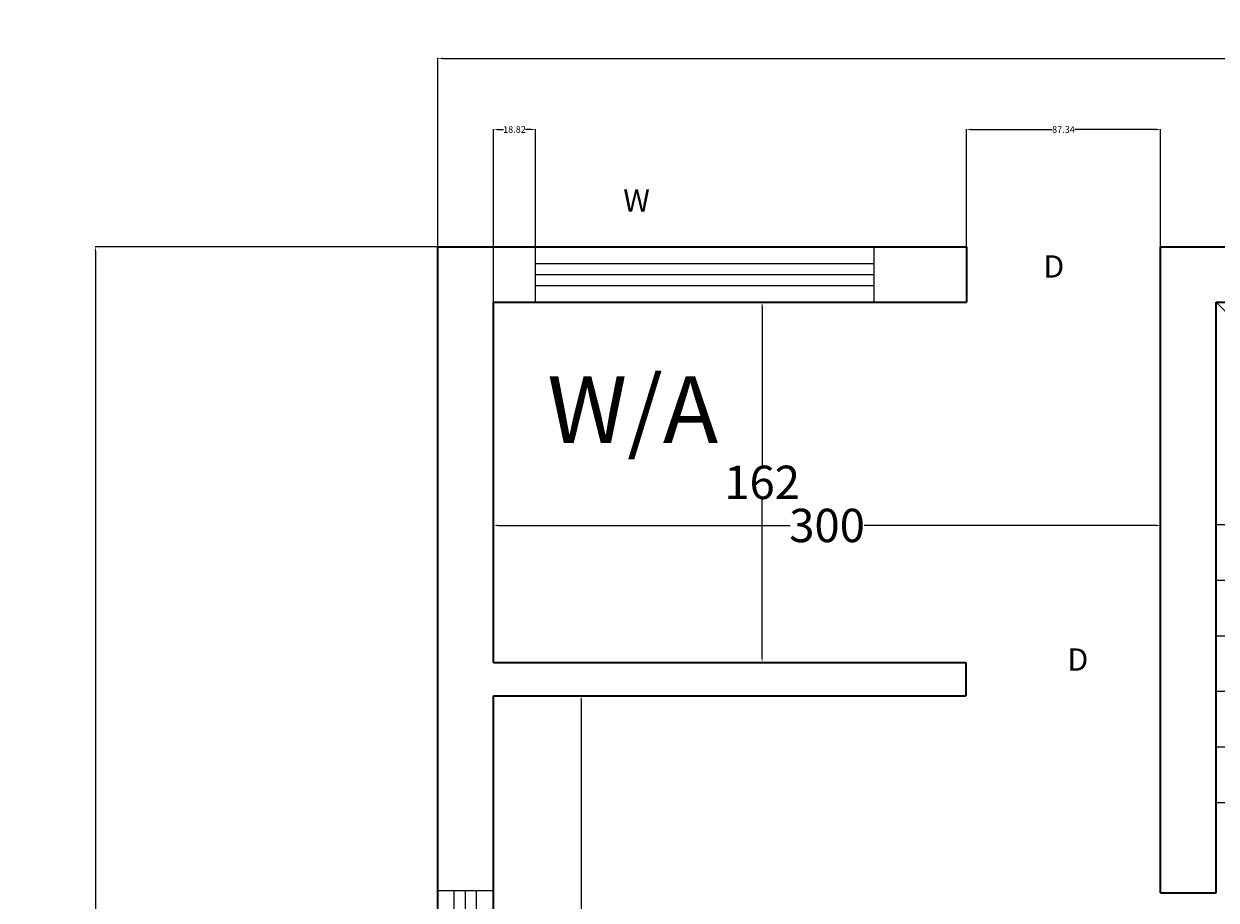
# Model space of a CAD drawing. Units: centimetres. Extents: x -121 to 3851, y -16 to 1180.
# Tile 4 of 16: x -121 to 415, y 586 to 980. Entities that reach past the tile are written whole.
import ezdxf

# ---------------------------------------------------------------- set-up
doc = ezdxf.new("R2010")
doc.units = ezdxf.units.CM
doc.header["$MEASUREMENT"] = 0
for name, color, linetype, lineweight in [('A-ANNO-DIMS', 2, 'Continuous', 18), ('A-ANNO-IDEN', 3, 'Continuous', 13), ('A-AREA-IDEN', 3, 'Continuous', 18), ('A-FLOR-STRS', 3, 'Continuous', 18), ('A-GLAZ', 4, 'Continuous', 18), ('A-WALL', 7, 'Continuous', 35)]:
    doc.layers.add(name, color=color, linetype=linetype, lineweight=lineweight)
doc.styles.get("Standard").update_dxf_attribs({"font": 'arial.ttf'})
doc.dimstyles.get("Standard").update_dxf_attribs({"dimtxt": 3, "dimasz": 2, "dimexe": 0.18, "dimexo": 0.0625, "dimgap": 0.09, "dimtad": 0, "dimtih": 1, "dimtoh": 1, "dimdec": 0, "dimzin": 0, "dimdsep": 46, "dimtxsty": 'Standard', "dimcen": 0.09, "dimadec": 0, "dimazin": 0, "dimtfac": 1, "dimtdec": 0, "dimtofl": 0, "dimtmove": 0, "dimatfit": 3, "dimfxl": 1, "dimtolj": 1, "dimtzin": 0, "dimarcsym": 0})

# ---------------------------------------------------------------- blocks, each defined once
blk = doc.blocks.new('*D1')
at = {"layer": 'A-ANNO-DIMS', "color": 0, "lineweight": -2, "transparency": 16777216}
for p, q in [((65.04, 880.08), (65.04, 964.95)), ((67.04, 964.77), (699.58, 964.77)), ((1419.04, 964.77), (786.5, 964.77)), ((1421.04, 880.08), (1421.04, 964.95))]:
    blk.add_line(p, q, dxfattribs=at)
at = {"layer": 'A-ANNO-DIMS', "color": 0, "transparency": 16777216}
for points in [[(67.04, 965.1), (67.04, 964.43), (65.04, 964.77)], [(1419.04, 965.1), (1419.04, 964.43), (1421.04, 964.77)]]:
    blk.add_solid(points, dxfattribs=at)
at = {"layer": 'Defpoints', "color": 0, "transparency": 16777216}
for p in [(1421.04, 964.77), (65.04, 880.01), (1421.04, 880.01)]:
    blk.add_point(p, dxfattribs=at)
at = {"layer": 'A-ANNO-DIMS', "color": 0, "transparency": 16777216, "insert": (743.04, 964.77), "char_height": 3, "attachment_point": 5}
blk.add_mtext('\\A1;{\\H10x;1356}', dxfattribs=at)
blk = doc.blocks.new('*D2')
at = {"layer": 'A-ANNO-DIMS', "color": 0, "lineweight": -2, "transparency": 16777216}
for p, q in [((64.98, 880.01), (-89.22, 880.01)), ((-89.04, 878.01), (-89.04, 487.42)), ((-89.04, 66.01), (-89.04, 456.61)), ((64.98, 64.01), (-89.22, 64.01))]:
    blk.add_line(p, q, dxfattribs=at)
at = {"layer": 'A-ANNO-DIMS', "color": 0, "transparency": 16777216}
for points in [[(-89.37, 878.01), (-88.71, 878.01), (-89.04, 880.01)], [(-89.37, 66.01), (-88.71, 66.01), (-89.04, 64.01)]]:
    blk.add_solid(points, dxfattribs=at)
at = {"layer": 'Defpoints', "color": 0, "transparency": 16777216}
for p in [(65.04, 880.01), (-89.04, 64.01), (65.04, 64.01)]:
    blk.add_point(p, dxfattribs=at)
at = {"layer": 'A-ANNO-DIMS', "color": 0, "transparency": 16777216, "insert": (-89.04, 472.01), "char_height": 3, "attachment_point": 5}
blk.add_mtext('\\A1;{\\H10x;816}', dxfattribs=at)
blk = doc.blocks.new('*D3')
at = {"layer": 'A-ANNO-DIMS', "color": 0, "lineweight": -2, "transparency": 16777216}
for p, q in [((185.01, 855.01), (211, 855.01)), ((210.82, 853.01), (210.82, 781.76)), ((210.82, 695.01), (210.82, 766.27)), ((185.01, 693.01), (211, 693.01))]:
    blk.add_line(p, q, dxfattribs=at)
at = {"layer": 'A-ANNO-DIMS', "color": 0, "transparency": 16777216}
for points in [[(210.48, 853.01), (211.15, 853.01), (210.82, 855.01)], [(210.48, 695.01), (211.15, 695.01), (210.82, 693.01)]]:
    blk.add_solid(points, dxfattribs=at)
at = {"layer": 'Defpoints', "color": 0, "transparency": 16777216}
for p in [(184.95, 855.01), (184.95, 693.01), (210.82, 693.01)]:
    blk.add_point(p, dxfattribs=at)
at = {"layer": 'A-ANNO-DIMS', "color": 0, "transparency": 16777216, "insert": (210.82, 774.01), "char_height": 3, "attachment_point": 5}
blk.add_mtext('\\A1;{\\H5x;162}', dxfattribs=at)
blk = doc.blocks.new('*D4')
at = {"layer": 'A-ANNO-DIMS', "color": 0, "lineweight": -2, "transparency": 16777216}
for p, q in [((90.04, 754.68), (90.04, 754.8)), ((92.04, 754.62), (223.41, 754.62)), ((388.04, 754.62), (256.67, 754.62)), ((390.04, 754.68), (390.04, 754.8))]:
    blk.add_line(p, q, dxfattribs=at)
at = {"layer": 'A-ANNO-DIMS', "color": 0, "transparency": 16777216}
for points in [[(92.04, 754.95), (92.04, 754.29), (90.04, 754.62)], [(388.04, 754.95), (388.04, 754.29), (390.04, 754.62)]]:
    blk.add_solid(points, dxfattribs=at)
at = {"layer": 'Defpoints', "color": 0, "transparency": 16777216}
for p in [(90.04, 754.62), (390.04, 754.62), (390.04, 754.62)]:
    blk.add_point(p, dxfattribs=at)
at = {"layer": 'A-ANNO-DIMS', "color": 0, "transparency": 16777216, "insert": (240.04, 754.62), "char_height": 3, "attachment_point": 5}
blk.add_mtext('\\A1;{\\H5x;300}', dxfattribs=at)
blk = doc.blocks.new('*D5')
at = {"layer": 'A-ANNO-DIMS', "color": 0, "lineweight": -2, "transparency": 16777216}
for p, q in [((196.17, 678.01), (129.29, 678.01)), ((129.47, 676.01), (129.47, 538.76)), ((129.47, 386.01), (129.47, 523.27)), ((196.17, 384.01), (129.29, 384.01))]:
    blk.add_line(p, q, dxfattribs=at)
at = {"layer": 'A-ANNO-DIMS', "color": 0, "transparency": 16777216}
for points in [[(129.13, 676.01), (129.8, 676.01), (129.47, 678.01)], [(129.13, 386.01), (129.8, 386.01), (129.47, 384.01)]]:
    blk.add_solid(points, dxfattribs=at)
at = {"layer": 'Defpoints', "color": 0, "transparency": 16777216}
for p in [(196.23, 678.01), (129.47, 384.01), (196.23, 384.01)]:
    blk.add_point(p, dxfattribs=at)
at = {"layer": 'A-ANNO-DIMS', "color": 0, "transparency": 16777216, "insert": (129.47, 531.01), "char_height": 3, "attachment_point": 5}
blk.add_mtext('\\A1;{\\H5x;294}', dxfattribs=at)
blk = doc.blocks.new('WIN-152CM')
for p, q in [((0, 17.5), (152.19, 17.5)), ((0, 12.5), (152.19, 12.5)), ((0, 7.5), (152.19, 7.5))]:
    blk.add_line(p, q)
blk.add_lwpolyline([(0, 25), (152.19, 25), (152.19, 0), (0, 0)], close=True)
blk = doc.blocks.new('STAIR-L-RETURN')
for p, q in [((0, 225), (99.13, 125)), ((100, 100), (100, 225)), ((125, 125), (125, 225)), ((150, 125), (150, 225)), ((175, 125), (175, 225)), ((200, 125), (200, 225)), ((225, 125), (225, 225)), ((250, 125), (250, 225)), ((275, 125), (275, 225)), ((0, 125), (99.13, 125)), ((99.13, 125), (354, 125)), ((100, 0), (100, 125)), ((0, 100), (100, 100)), ((0, 75), (100, 75)), ((0, 50), (100, 50)), ((0, 25), (100, 25)), ((0, 0), (100, 0))]:
    blk.add_line(p, q)
blk = doc.blocks.new('*D41')
at = {"layer": 'A-ANNO-DIMS', "color": 0, "lineweight": -2, "transparency": 16777216}
for p, q in [((302.7, 855.08), (302.7, 932.94)), ((304.7, 932.76), (341.22, 932.76)), ((388.04, 932.76), (351.52, 932.76)), ((390.04, 855.08), (390.04, 932.94))]:
    blk.add_line(p, q, dxfattribs=at)
at = {"layer": 'A-ANNO-DIMS', "color": 0, "transparency": 16777216}
for points in [[(304.7, 933.1), (304.7, 932.43), (302.7, 932.76)], [(388.04, 933.1), (388.04, 932.43), (390.04, 932.76)]]:
    blk.add_solid(points, dxfattribs=at)
at = {"layer": 'Defpoints', "color": 0, "transparency": 16777216}
for p in [(390.04, 932.76), (302.7, 855.01), (390.04, 855.01)]:
    blk.add_point(p, dxfattribs=at)
at = {"layer": 'A-ANNO-DIMS', "color": 0, "transparency": 16777216, "insert": (346.37, 932.76), "char_height": 3, "attachment_point": 5}
blk.add_mtext('\\A1;87.34', dxfattribs=at)
blk = doc.blocks.new('*D42')
at = {"layer": 'A-ANNO-DIMS', "color": 0, "lineweight": -2, "transparency": 16777216}
for p, q in [((90.04, 855.08), (90.04, 932.94)), ((92.04, 932.76), (94.45, 932.76)), ((106.86, 932.76), (104.44, 932.76)), ((108.86, 855.08), (108.86, 932.94))]:
    blk.add_line(p, q, dxfattribs=at)
at = {"layer": 'A-ANNO-DIMS', "color": 0, "transparency": 16777216}
for points in [[(92.04, 933.1), (92.04, 932.43), (90.04, 932.76)], [(106.86, 933.1), (106.86, 932.43), (108.86, 932.76)]]:
    blk.add_solid(points, dxfattribs=at)
at = {"layer": 'Defpoints', "color": 0, "transparency": 16777216}
for p in [(108.86, 932.76), (90.04, 855.01), (108.86, 855.01)]:
    blk.add_point(p, dxfattribs=at)
at = {"layer": 'A-ANNO-DIMS', "color": 0, "transparency": 16777216, "insert": (99.45, 932.76), "char_height": 3, "attachment_point": 5}
blk.add_mtext('\\A1;18.82', dxfattribs=at)

msp = doc.modelspace()

# ---------------------------------------------------------------- linework, layer by layer
at = {"layer": 'A-WALL'}
for p, q in [((65.0382, 880.0141), (302.6973, 880.0141)), ((65.0382, 64.0141), (65.0382, 880.0141)), ((302.6973, 880.0141), (302.6973, 855.0141)), ((390.0382, 855.0141), (390.0382, 880.0141)), ((390.0382, 880.0141), (1421.0382, 880.0141)), ((90.0382, 855.0141), (302.6973, 855.0141)), ((90.0382, 693.0141), (90.0382, 855.0141)), ((390.0382, 678.0141), (390.0382, 855.0141)), ((415.0382, 589.2848), (415.0382, 855.0141)), ((415.0382, 855.0141), (769.0382, 855.0141)), ((90.0382, 693.0141), (302.4175, 693.0141)), ((302.4175, 693.0141), (302.4175, 678.0141)), ((90.0382, 678.0141), (302.4175, 678.0141)), ((90.0382, 358.0141), (90.0382, 678.0141)), ((390.0382, 589.2848), (390.0382, 678.0141)), ((390.0382, 589.2848), (415.0382, 589.2848))]:
    msp.add_line(p, q, dxfattribs=at)

# ---------------------------------------------------------------- block references
at = {"layer": 'A-FLOR-STRS'}
msp.add_blockref('STAIR-L-RETURN', (415.038, 630.014), dxfattribs=at)
at = {"layer": 'A-GLAZ'}
msp.add_blockref('WIN-152CM', (108.857, 855.014), dxfattribs=at)
at = {"layer": 'A-GLAZ', "rotation": 89.99999999999991}
msp.add_blockref('WIN-152CM', (89.8847, 438.1982), dxfattribs=at)

# ---------------------------------------------------------------- texts
at = {"layer": 'A-ANNO-IDEN', "char_height": 10, "attachment_point": 1}
for s, insert in [('W', (148.3632, 905.8062)), ('D', (337.3118, 876.1426)), ('D', (348.1435, 699.2905))]:
    msp.add_mtext_dynamic_manual_height_columns(s, width=55.718495, gutter_width=1, heights=[0], dxfattribs=dict(at, insert=insert))
at = {"layer": 'A-AREA-IDEN', "insert": (114.1959, 821.7126), "char_height": 30, "attachment_point": 1}
msp.add_mtext_dynamic_manual_height_columns('W/A', width=114.805391, gutter_width=1, heights=[0], dxfattribs=at)

# ---------------------------------------------------------------- dimensions: what is measured, and where the dimension line sits
at = {"layer": 'A-ANNO-DIMS'}
for base, p1, p2, text, picture, middle in [((1421.0382, 964.7682), (65.0382, 880.0141), (1421.0382, 880.0141), '{\\H10x;<>}', '*D1', (743.0382, 964.7682)), ((390.0382, 754.6211), (90.0382, 754.6211), (390.0382, 754.6211), '{\\H5x;<>}', '*D4', (240.0382, 754.6211))]:
    dim = msp.add_linear_dim(base=base, p1=p1, p2=p2, text=text, dimstyle='Standard', override={"dimclrd": 0, "dimclre": 0, "dimclrt": 0}, dxfattribs=at)
    dim.commit()
    dim.dimension.update_dxf_attribs({"geometry": picture, "text_midpoint": middle})
for base, p1, p2, picture, middle in [((108.8571, 932.7641), (90.0382, 855.0141), (108.8571, 855.0141), '*D42', (99.4477, 932.7641)), ((390.0382, 932.7641), (302.6973, 855.0141), (390.0382, 855.0141), '*D41', (346.3678, 932.7641))]:
    dim = msp.add_linear_dim(base=base, p1=p1, p2=p2, dimstyle='Standard', override={"dimdec": 2, "dimlfac": 1, "dimrnd": 0, "dimzin": 0, "dimdsep": 46, "dimlunit": 2}, dxfattribs=at)
    dim.commit()
    dim.dimension.update_dxf_attribs({"geometry": picture, "text_midpoint": middle})
for base, p1, p2, text, picture, middle in [((-89.041, 64.0141), (65.0382, 880.0141), (65.0382, 64.0141), '{\\H10x;<>}', '*D2', (-89.041, 472.0141)), ((210.8183, 693.0141), (184.9523, 855.0141), (184.9523, 693.0141), '{\\H5x;<>}', '*D3', (210.8183, 774.0141)), ((129.4663, 384.0141), (196.2278, 678.0141), (196.2278, 384.0141), '{\\H5x;<>}', '*D5', (129.4663, 531.0141))]:
    dim = msp.add_linear_dim(base=base, p1=p1, p2=p2, angle=90, text=text, dimstyle='Standard', override={"dimclrd": 0, "dimclre": 0, "dimclrt": 0}, dxfattribs=at)
    dim.commit()
    dim.dimension.update_dxf_attribs({"geometry": picture, "text_midpoint": middle})

doc.saveas('drawing.dxf')
